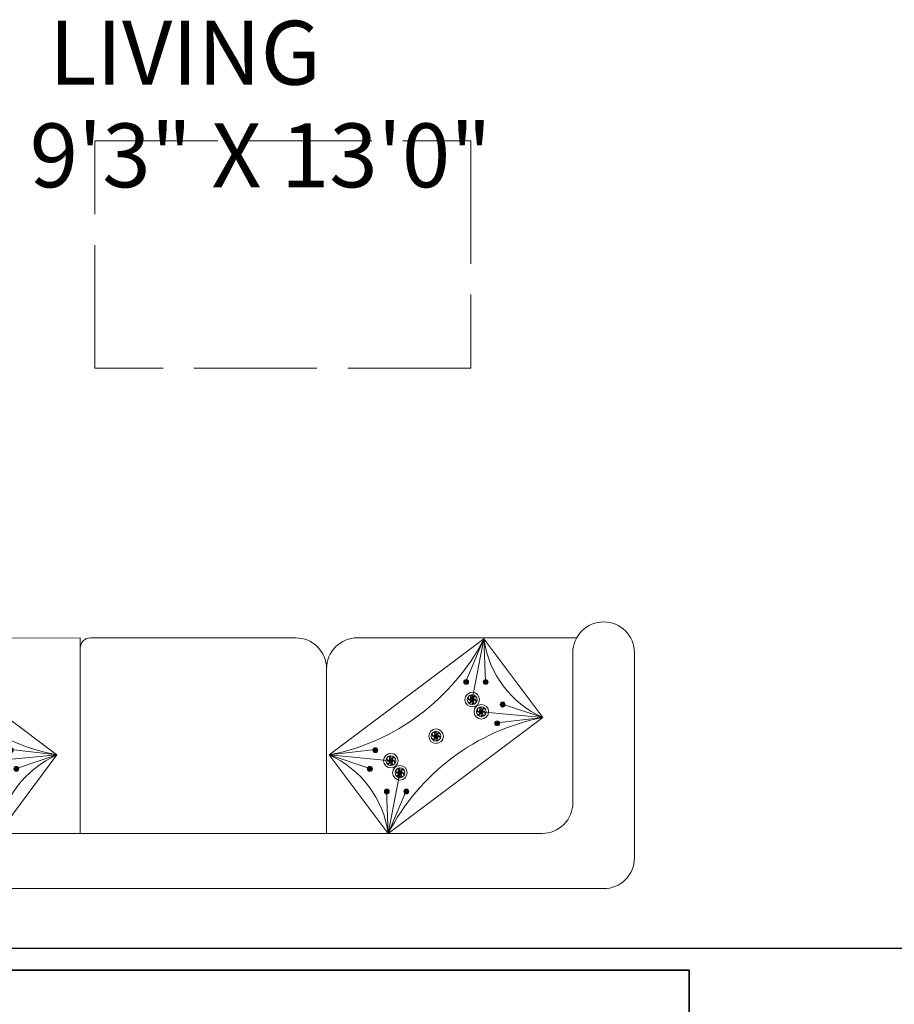
# Model space of a CAD drawing. Units: inches. Extents: x -61 to 1599, y -1316 to 257.
# Tile 194 of 204: x 1147 to 1233, y -173 to -77. Entities that reach past the tile are written whole.
import ezdxf

# ---------------------------------------------------------------- set-up
doc = ezdxf.new("R2010")
doc.units = ezdxf.units.IN
doc.header["$MEASUREMENT"] = 0
doc.linetypes.add('ACAD_ISO02W100', pattern=[15, 12, -3])
for name, color, linetype, lineweight in [('A-ANNO-DIMS', 2, 'Continuous', 18), ('A-AREA-IDEN', 1, 'Continuous', 18), ('A-FURN-LOW', 83, 'ACAD_ISO02W100', 18), ('FURNITURE', 83, 'Continuous', 18), ('WALLS', 4, 'Continuous', 35)]:
    doc.layers.add(name, color=color, linetype=linetype, lineweight=lineweight)
doc.layers.add('FUR', color=83, linetype='Continuous')
doc.styles.get("Standard").update_dxf_attribs({"font": 'arial.ttf'})
doc.dimstyles.get("Standard").update_dxf_attribs({"dimtxt": 0.18, "dimasz": 0.18, "dimexe": 0.18, "dimexo": 0.0625, "dimgap": 0.09, "dimtad": 0, "dimtih": 1, "dimtoh": 1, "dimdec": 0, "dimzin": 0, "dimdsep": 46, "dimlunit": 3, "dimtxsty": 'Standard', "dimcen": 0.09, "dimadec": 0, "dimazin": 0, "dimtfac": 1, "dimtdec": 0, "dimtofl": 0, "dimtmove": 0, "dimatfit": 3, "dimfxl": 1, "dimtolj": 1, "dimtzin": 0, "dimarcsym": 0})

# ---------------------------------------------------------------- blocks, each defined once
blk = doc.blocks.new('*U152')
at = {"layer": 'FUR'}
blk.add_open_spline([(0.005, 0.08), (-0.03, 0.048), (-0.098, -0.015), (0.075, -0.018), (0.024, -0.063), (0.005, -0.08)], degree=3, knots=[0, 0, 0, 0, 0.0954578, 0.1898773, 0.2470677, 0.2470677, 0.2470677, 0.2470677], dxfattribs=at)
blk = doc.blocks.new('*U153')
at = {"layer": 'FUR', "transparency": 16777216}
for p, rotation in [((222.173, -79.977), 60), ((222.178, -80.056), 120), ((222.25, -80.092), 180), ((222.312, -79.968), 300), ((222.317, -80.048), 240)]:
    blk.add_blockref('*U152', p, dxfattribs=dict(at, rotation=rotation))
blk.add_blockref('*U152', (222.24, -79.932), dxfattribs=at)
blk = doc.blocks.new('*U154')
at = {"layer": 'FUR'}
blk.add_open_spline([(0.005, 0.08), (-0.03, 0.048), (-0.098, -0.015), (0.075, -0.018), (0.024, -0.063), (0.005, -0.08)], degree=3, knots=[0, 0, 0, 0, 0.0954578, 0.1898773, 0.2470677, 0.2470677, 0.2470677, 0.2470677], dxfattribs=at)
blk = doc.blocks.new('*U155')
at = {"layer": 'FUR', "transparency": 16777216}
for p, rotation in [((222.173, -79.977), 60), ((222.178, -80.056), 120), ((222.25, -80.092), 180), ((222.312, -79.968), 300), ((222.317, -80.048), 240)]:
    blk.add_blockref('*U154', p, dxfattribs=dict(at, rotation=rotation))
blk.add_blockref('*U154', (222.24, -79.932), dxfattribs=at)
blk = doc.blocks.new('*U148')
at = {"layer": 'FUR'}
blk.add_open_spline([(0.005, 0.08), (-0.03, 0.048), (-0.098, -0.015), (0.075, -0.018), (0.024, -0.063), (0.005, -0.08)], degree=3, knots=[0, 0, 0, 0, 0.0954578, 0.1898773, 0.2470677, 0.2470677, 0.2470677, 0.2470677], dxfattribs=at)
blk = doc.blocks.new('*U149')
at = {"layer": 'FUR', "transparency": 16777216}
for p, rotation in [((222.173, -79.977), 60), ((222.178, -80.056), 120), ((222.25, -80.092), 180), ((222.312, -79.968), 300), ((222.317, -80.048), 240)]:
    blk.add_blockref('*U148', p, dxfattribs=dict(at, rotation=rotation))
blk.add_blockref('*U148', (222.24, -79.932), dxfattribs=at)
blk = doc.blocks.new('*U128')
at = {"layer": 'FUR'}
blk.add_open_spline([(0.015, 0.238), (-0.088, 0.143), (-0.292, -0.045), (0.224, -0.053), (0.072, -0.187), (0.015, -0.238)], degree=3, knots=[0, 0, 0, 0, 0.2846533, 0.5662105, 0.736751, 0.736751, 0.736751, 0.736751], dxfattribs=at)
blk = doc.blocks.new('*U129')
at = {"layer": 'FUR', "transparency": 16777216}
for p, rotation in [((662.517, -238.489), 60), ((662.531, -238.727), 120), ((662.745, -238.833), 180), ((662.929, -238.463), 300), ((662.944, -238.702), 240)]:
    blk.add_blockref('*U128', p, dxfattribs=dict(at, rotation=rotation))
blk.add_blockref('*U128', (662.716, -238.357), dxfattribs=at)
blk = doc.blocks.new('*U150')
at = {"layer": 'FUR'}
blk.add_open_spline([(0.005, 0.08), (-0.03, 0.048), (-0.098, -0.015), (0.075, -0.018), (0.024, -0.063), (0.005, -0.08)], degree=3, knots=[0, 0, 0, 0, 0.0954578, 0.1898773, 0.2470677, 0.2470677, 0.2470677, 0.2470677], dxfattribs=at)
blk = doc.blocks.new('*U151')
at = {"layer": 'FUR', "transparency": 16777216}
for p, rotation in [((222.173, -79.977), 60), ((222.178, -80.056), 120), ((222.25, -80.092), 180), ((222.312, -79.968), 300), ((222.317, -80.048), 240)]:
    blk.add_blockref('*U150', p, dxfattribs=dict(at, rotation=rotation))
blk.add_blockref('*U150', (222.24, -79.932), dxfattribs=at)
blk = doc.blocks.new('*U132')
at = {"layer": 'FUR'}
blk.add_open_spline([(0.015, 0.238), (-0.088, 0.143), (-0.292, -0.045), (0.224, -0.053), (0.072, -0.187), (0.015, -0.238)], degree=3, knots=[0, 0, 0, 0, 0.2846533, 0.5662105, 0.736751, 0.736751, 0.736751, 0.736751], dxfattribs=at)
blk = doc.blocks.new('*U133')
at = {"layer": 'FUR', "transparency": 16777216}
for p, rotation in [((662.517, -238.489), 60), ((662.531, -238.727), 120), ((662.745, -238.833), 180), ((662.929, -238.463), 300), ((662.944, -238.702), 240)]:
    blk.add_blockref('*U132', p, dxfattribs=dict(at, rotation=rotation))
blk.add_blockref('*U132', (662.716, -238.357), dxfattribs=at)
blk = doc.blocks.new('*U124')
at = {"layer": 'FUR'}
blk.add_open_spline([(0.005, 0.08), (-0.03, 0.048), (-0.098, -0.015), (0.075, -0.018), (0.024, -0.063), (0.005, -0.08)], degree=3, knots=[0, 0, 0, 0, 0.0954578, 0.1898773, 0.2470677, 0.2470677, 0.2470677, 0.2470677], dxfattribs=at)
blk = doc.blocks.new('*U125')
at = {"layer": 'FUR', "transparency": 16777216}
for p, rotation in [((222.173, -79.977), 60), ((222.178, -80.056), 120), ((222.25, -80.092), 180), ((222.312, -79.968), 300), ((222.317, -80.048), 240)]:
    blk.add_blockref('*U124', p, dxfattribs=dict(at, rotation=rotation))
blk.add_blockref('*U124', (222.24, -79.932), dxfattribs=at)
blk = doc.blocks.new('*U134')
at = {"layer": 'FUR'}
blk.add_open_spline([(0.015, 0.238), (-0.088, 0.143), (-0.292, -0.045), (0.224, -0.053), (0.072, -0.187), (0.015, -0.238)], degree=3, knots=[0, 0, 0, 0, 0.2846533, 0.5662105, 0.736751, 0.736751, 0.736751, 0.736751], dxfattribs=at)
blk = doc.blocks.new('*U123')
at = {"layer": 'FUR', "transparency": 16777216}
for p, rotation in [((662.517, -238.489), 60), ((662.531, -238.727), 120), ((662.745, -238.833), 180), ((662.929, -238.463), 300), ((662.944, -238.702), 240)]:
    blk.add_blockref('*U134', p, dxfattribs=dict(at, rotation=rotation))
blk.add_blockref('*U134', (662.716, -238.357), dxfattribs=at)
blk = doc.blocks.new('*U130')
at = {"layer": 'FUR'}
blk.add_open_spline([(0.015, 0.238), (-0.088, 0.143), (-0.292, -0.045), (0.224, -0.053), (0.072, -0.187), (0.015, -0.238)], degree=3, knots=[0, 0, 0, 0, 0.2846533, 0.5662105, 0.736751, 0.736751, 0.736751, 0.736751], dxfattribs=at)
blk = doc.blocks.new('*U131')
at = {"layer": 'FUR', "transparency": 16777216}
for p, rotation in [((662.517, -238.489), 60), ((662.531, -238.727), 120), ((662.745, -238.833), 180), ((662.929, -238.463), 300), ((662.944, -238.702), 240)]:
    blk.add_blockref('*U130', p, dxfattribs=dict(at, rotation=rotation))
blk.add_blockref('*U130', (662.716, -238.357), dxfattribs=at)
blk = doc.blocks.new('*U126')
at = {"layer": 'FUR'}
blk.add_open_spline([(0.005, 0.08), (-0.03, 0.048), (-0.098, -0.015), (0.075, -0.018), (0.024, -0.063), (0.005, -0.08)], degree=3, knots=[0, 0, 0, 0, 0.0954578, 0.1898773, 0.2470677, 0.2470677, 0.2470677, 0.2470677], dxfattribs=at)
blk = doc.blocks.new('*U127')
at = {"layer": 'FUR', "transparency": 16777216}
for p, rotation in [((222.173, -79.977), 60), ((222.178, -80.056), 120), ((222.25, -80.092), 180), ((222.312, -79.968), 300), ((222.317, -80.048), 240)]:
    blk.add_blockref('*U126', p, dxfattribs=dict(at, rotation=rotation))
blk.add_blockref('*U126', (222.24, -79.932), dxfattribs=at)
blk = doc.blocks.new('*U146')
at = {"layer": 'FUR'}
blk.add_open_spline([(0.005, 0.08), (-0.03, 0.048), (-0.098, -0.015), (0.075, -0.018), (0.024, -0.063), (0.005, -0.08)], degree=3, knots=[0, 0, 0, 0, 0.0954578, 0.1898773, 0.2470677, 0.2470677, 0.2470677, 0.2470677], dxfattribs=at)
blk = doc.blocks.new('*U147')
at = {"layer": 'FUR', "transparency": 16777216}
for p, rotation in [((222.173, -79.977), 60), ((222.178, -80.056), 120), ((222.25, -80.092), 180), ((222.312, -79.968), 300), ((222.317, -80.048), 240)]:
    blk.add_blockref('*U146', p, dxfattribs=dict(at, rotation=rotation))
blk.add_blockref('*U146', (222.24, -79.932), dxfattribs=at)
blk = doc.blocks.new('*U144')
at = {"layer": 'FUR'}
blk.add_open_spline([(0.005, 0.08), (-0.03, 0.048), (-0.098, -0.015), (0.075, -0.018), (0.024, -0.063), (0.005, -0.08)], degree=3, knots=[0, 0, 0, 0, 0.0954578, 0.1898773, 0.2470677, 0.2470677, 0.2470677, 0.2470677], dxfattribs=at)
blk = doc.blocks.new('*U145')
at = {"layer": 'FUR', "transparency": 16777216}
for p, rotation in [((222.173, -79.977), 60), ((222.178, -80.056), 120), ((222.25, -80.092), 180), ((222.312, -79.968), 300), ((222.317, -80.048), 240)]:
    blk.add_blockref('*U144', p, dxfattribs=dict(at, rotation=rotation))
blk.add_blockref('*U144', (222.24, -79.932), dxfattribs=at)
blk = doc.blocks.new('*U114')
at = {"layer": 'FUR'}
blk.add_open_spline([(0.005, 0.08), (-0.03, 0.048), (-0.098, -0.015), (0.075, -0.018), (0.024, -0.063), (0.005, -0.08)], degree=3, knots=[0, 0, 0, 0, 0.0954578, 0.1898773, 0.2470677, 0.2470677, 0.2470677, 0.2470677], dxfattribs=at)
blk = doc.blocks.new('*U115')
at = {"layer": 'FUR', "transparency": 16777216}
for p, rotation in [((222.173, -79.977), 60), ((222.178, -80.056), 120), ((222.25, -80.092), 180), ((222.312, -79.968), 300), ((222.317, -80.048), 240)]:
    blk.add_blockref('*U114', p, dxfattribs=dict(at, rotation=rotation))
blk.add_blockref('*U114', (222.24, -79.932), dxfattribs=at)
blk = doc.blocks.new('*U116')
at = {"layer": 'FUR'}
blk.add_open_spline([(0.005, 0.08), (-0.03, 0.048), (-0.098, -0.015), (0.075, -0.018), (0.024, -0.063), (0.005, -0.08)], degree=3, knots=[0, 0, 0, 0, 0.0954578, 0.1898773, 0.2470677, 0.2470677, 0.2470677, 0.2470677], dxfattribs=at)
blk = doc.blocks.new('*U117')
at = {"layer": 'FUR', "transparency": 16777216}
for p, rotation in [((222.173, -79.977), 60), ((222.178, -80.056), 120), ((222.25, -80.092), 180), ((222.312, -79.968), 300), ((222.317, -80.048), 240)]:
    blk.add_blockref('*U116', p, dxfattribs=dict(at, rotation=rotation))
blk.add_blockref('*U116', (222.24, -79.932), dxfattribs=at)
blk = doc.blocks.new('*U112')
at = {"layer": 'FUR'}
blk.add_open_spline([(0.005, 0.08), (-0.03, 0.048), (-0.098, -0.015), (0.075, -0.018), (0.024, -0.063), (0.005, -0.08)], degree=3, knots=[0, 0, 0, 0, 0.0954578, 0.1898773, 0.2470677, 0.2470677, 0.2470677, 0.2470677], dxfattribs=at)
blk = doc.blocks.new('*U113')
at = {"layer": 'FUR', "transparency": 16777216}
for p, rotation in [((222.173, -79.977), 60), ((222.178, -80.056), 120), ((222.25, -80.092), 180), ((222.312, -79.968), 300), ((222.317, -80.048), 240)]:
    blk.add_blockref('*U112', p, dxfattribs=dict(at, rotation=rotation))
blk.add_blockref('*U112', (222.24, -79.932), dxfattribs=at)
blk = doc.blocks.new('*U142')
at = {"layer": 'FUR'}
blk.add_open_spline([(0.015, 0.238), (-0.088, 0.143), (-0.292, -0.045), (0.224, -0.053), (0.072, -0.187), (0.015, -0.238)], degree=3, knots=[0, 0, 0, 0, 0.2846533, 0.5662105, 0.736751, 0.736751, 0.736751, 0.736751], dxfattribs=at)
blk = doc.blocks.new('*U143')
at = {"layer": 'FUR', "transparency": 16777216}
for p, rotation in [((662.517, -238.489), 60), ((662.531, -238.727), 120), ((662.745, -238.833), 180), ((662.929, -238.463), 300), ((662.944, -238.702), 240)]:
    blk.add_blockref('*U142', p, dxfattribs=dict(at, rotation=rotation))
blk.add_blockref('*U142', (662.716, -238.357), dxfattribs=at)
blk = doc.blocks.new('*U158')
at = {"layer": 'FUR'}
blk.add_open_spline([(0.015, 0.238), (-0.088, 0.143), (-0.292, -0.045), (0.224, -0.053), (0.072, -0.187), (0.015, -0.238)], degree=3, knots=[0, 0, 0, 0, 0.2846533, 0.5662105, 0.736751, 0.736751, 0.736751, 0.736751], dxfattribs=at)
blk = doc.blocks.new('*U109')
at = {"layer": 'FUR', "transparency": 16777216}
for p, rotation in [((662.517, -238.489), 60), ((662.531, -238.727), 120), ((662.745, -238.833), 180), ((662.929, -238.463), 300), ((662.944, -238.702), 240)]:
    blk.add_blockref('*U158', p, dxfattribs=dict(at, rotation=rotation))
blk.add_blockref('*U158', (662.716, -238.357), dxfattribs=at)
blk = doc.blocks.new('*U110')
at = {"layer": 'FUR'}
blk.add_open_spline([(0.005, 0.08), (-0.03, 0.048), (-0.098, -0.015), (0.075, -0.018), (0.024, -0.063), (0.005, -0.08)], degree=3, knots=[0, 0, 0, 0, 0.0954578, 0.1898773, 0.2470677, 0.2470677, 0.2470677, 0.2470677], dxfattribs=at)
blk = doc.blocks.new('*U111')
at = {"layer": 'FUR', "transparency": 16777216}
for p, rotation in [((222.173, -79.977), 60), ((222.178, -80.056), 120), ((222.25, -80.092), 180), ((222.312, -79.968), 300), ((222.317, -80.048), 240)]:
    blk.add_blockref('*U110', p, dxfattribs=dict(at, rotation=rotation))
blk.add_blockref('*U110', (222.24, -79.932), dxfattribs=at)
blk = doc.blocks.new('*U156')
at = {"layer": 'FUR'}
blk.add_open_spline([(0.015, 0.238), (-0.088, 0.143), (-0.292, -0.045), (0.224, -0.053), (0.072, -0.187), (0.015, -0.238)], degree=3, knots=[0, 0, 0, 0, 0.2846533, 0.5662105, 0.736751, 0.736751, 0.736751, 0.736751], dxfattribs=at)
blk = doc.blocks.new('*U157')
at = {"layer": 'FUR', "transparency": 16777216}
for p, rotation in [((662.517, -238.489), 60), ((662.531, -238.727), 120), ((662.745, -238.833), 180), ((662.929, -238.463), 300), ((662.944, -238.702), 240)]:
    blk.add_blockref('*U156', p, dxfattribs=dict(at, rotation=rotation))
blk.add_blockref('*U156', (662.716, -238.357), dxfattribs=at)
blk = doc.blocks.new('*U120')
at = {"layer": 'FUR'}
blk.add_open_spline([(0.005, 0.08), (-0.03, 0.048), (-0.098, -0.015), (0.075, -0.018), (0.024, -0.063), (0.005, -0.08)], degree=3, knots=[0, 0, 0, 0, 0.0954578, 0.1898773, 0.2470677, 0.2470677, 0.2470677, 0.2470677], dxfattribs=at)
blk = doc.blocks.new('*U121')
at = {"layer": 'FUR', "transparency": 16777216}
for p, rotation in [((222.173, -79.977), 60), ((222.178, -80.056), 120), ((222.25, -80.092), 180), ((222.312, -79.968), 300), ((222.317, -80.048), 240)]:
    blk.add_blockref('*U120', p, dxfattribs=dict(at, rotation=rotation))
blk.add_blockref('*U120', (222.24, -79.932), dxfattribs=at)
blk = doc.blocks.new('*U140')
at = {"layer": 'FUR'}
blk.add_open_spline([(0.015, 0.238), (-0.088, 0.143), (-0.292, -0.045), (0.224, -0.053), (0.072, -0.187), (0.015, -0.238)], degree=3, knots=[0, 0, 0, 0, 0.2846533, 0.5662105, 0.736751, 0.736751, 0.736751, 0.736751], dxfattribs=at)
blk = doc.blocks.new('*U141')
at = {"layer": 'FUR', "transparency": 16777216}
for p, rotation in [((662.517, -238.489), 60), ((662.531, -238.727), 120), ((662.745, -238.833), 180), ((662.929, -238.463), 300), ((662.944, -238.702), 240)]:
    blk.add_blockref('*U140', p, dxfattribs=dict(at, rotation=rotation))
blk.add_blockref('*U140', (662.716, -238.357), dxfattribs=at)
blk = doc.blocks.new('*U135')
at = {"layer": 'FUR'}
blk.add_open_spline([(0.015, 0.238), (-0.088, 0.143), (-0.292, -0.045), (0.224, -0.053), (0.072, -0.187), (0.015, -0.238)], degree=3, knots=[0, 0, 0, 0, 0.2846533, 0.5662105, 0.736751, 0.736751, 0.736751, 0.736751], dxfattribs=at)
blk = doc.blocks.new('*U136')
at = {"layer": 'FUR', "transparency": 16777216}
for p, rotation in [((662.517, -238.489), 60), ((662.531, -238.727), 120), ((662.745, -238.833), 180), ((662.929, -238.463), 300), ((662.944, -238.702), 240)]:
    blk.add_blockref('*U135', p, dxfattribs=dict(at, rotation=rotation))
blk.add_blockref('*U135', (662.716, -238.357), dxfattribs=at)
blk = doc.blocks.new('*U118')
at = {"layer": 'FUR'}
blk.add_open_spline([(0.005, 0.08), (-0.03, 0.048), (-0.098, -0.015), (0.075, -0.018), (0.024, -0.063), (0.005, -0.08)], degree=3, knots=[0, 0, 0, 0, 0.0954578, 0.1898773, 0.2470677, 0.2470677, 0.2470677, 0.2470677], dxfattribs=at)
blk = doc.blocks.new('*U119')
at = {"layer": 'FUR', "transparency": 16777216}
for p, rotation in [((222.173, -79.977), 60), ((222.178, -80.056), 120), ((222.25, -80.092), 180), ((222.312, -79.968), 300), ((222.317, -80.048), 240)]:
    blk.add_blockref('*U118', p, dxfattribs=dict(at, rotation=rotation))
blk.add_blockref('*U118', (222.24, -79.932), dxfattribs=at)
blk = doc.blocks.new('*U138')
at = {"layer": 'FUR'}
blk.add_open_spline([(0.005, 0.08), (-0.03, 0.048), (-0.098, -0.015), (0.075, -0.018), (0.024, -0.063), (0.005, -0.08)], degree=3, knots=[0, 0, 0, 0, 0.0954578, 0.1898773, 0.2470677, 0.2470677, 0.2470677, 0.2470677], dxfattribs=at)
blk = doc.blocks.new('*U139')
at = {"layer": 'FUR', "transparency": 16777216}
for p, rotation in [((222.173, -79.977), 60), ((222.178, -80.056), 120), ((222.25, -80.092), 180), ((222.312, -79.968), 300), ((222.317, -80.048), 240)]:
    blk.add_blockref('*U138', p, dxfattribs=dict(at, rotation=rotation))
blk.add_blockref('*U138', (222.24, -79.932), dxfattribs=at)
blk = doc.blocks.new('*U122')
at = {"layer": 'FUR'}
blk.add_open_spline([(0.005, 0.08), (-0.03, 0.048), (-0.098, -0.015), (0.075, -0.018), (0.024, -0.063), (0.005, -0.08)], degree=3, knots=[0, 0, 0, 0, 0.0954578, 0.1898773, 0.2470677, 0.2470677, 0.2470677, 0.2470677], dxfattribs=at)
blk = doc.blocks.new('*U137')
at = {"layer": 'FUR', "transparency": 16777216}
for p, rotation in [((222.173, -79.977), 60), ((222.178, -80.056), 120), ((222.25, -80.092), 180), ((222.312, -79.968), 300), ((222.317, -80.048), 240)]:
    blk.add_blockref('*U122', p, dxfattribs=dict(at, rotation=rotation))
blk.add_blockref('*U122', (222.24, -79.932), dxfattribs=at)
blk = doc.blocks.new('SOFA-THREE-SEAT')
for p, q in [((30, 24.442), (6.996, 24.38)), ((12.664, 24.333), (12.509, 20.192)), ((12.664, 24.333), (13.805, 18.423)), ((12.664, 24.333), (14.414, 20.192)), ((30, 23.442), (29.997, 24.442)), ((51, 24.442), (31, 24.442)), ((78.369, 24.442), (57, 24.442)), ((69.336, 24.333), (67.586, 20.192)), ((69.336, 24.333), (68.194, 18.423)), ((69.336, 24.333), (69.49, 20.192)), ((6, 23), (5.999, 23.377)), ((30, 23.442), (30, 5.382)), ((54, 21.442), (54, 5.382)), ((54, 21.442), (54, 21.442)), ((12.49, 20.139), (12.49, 20.299)), ((14.394, 20.139), (14.394, 20.299)), ((67.605, 20.139), (67.605, 20.299)), ((69.509, 20.139), (69.509, 20.299)), ((12.49, 20.139), (12.49, 19.979)), ((14.394, 20.139), (14.394, 19.979)), ((67.605, 20.139), (67.605, 19.979)), ((69.509, 20.139), (69.509, 19.979)), ((13.805, 18.423), (13.805, 18.899)), ((13.805, 18.423), (13.805, 17.946)), ((68.194, 18.423), (68.194, 18.899)), ((68.194, 18.423), (68.194, 17.946)), ((6.926, 16.687), (10.859, 17.993)), ((10.84, 17.94), (10.84, 18.1)), ((10.84, 17.94), (10.84, 17.78)), ((69.079, 17.243), (69.079, 17.719)), ((75.074, 16.687), (71.14, 17.993)), ((71.159, 17.94), (71.159, 18.1)), ((71.159, 17.94), (71.159, 17.78)), ((6.926, 16.687), (12.92, 17.243)), ((6.926, 16.687), (11.391, 16.164)), ((75.074, 16.687), (69.079, 17.243)), ((69.079, 17.243), (69.079, 16.766)), ((75.074, 16.687), (70.608, 16.164)), ((11.372, 16.112), (11.372, 16.272)), ((11.372, 16.112), (11.372, 15.952)), ((70.627, 16.112), (70.627, 16.272)), ((70.627, 16.112), (70.627, 15.952)), ((17.327, 14.857), (17.327, 15.334)), ((17.327, 14.857), (17.327, 14.381)), ((64.672, 14.857), (64.672, 15.334)), ((64.672, 14.857), (64.672, 14.381)), ((23.243, 13.498), (23.243, 13.658)), ((23.243, 13.498), (23.243, 13.338)), ((27.729, 13.028), (23.263, 13.551)), ((54.271, 13.028), (58.736, 13.551)), ((58.756, 13.498), (58.756, 13.658)), ((58.756, 13.498), (58.756, 13.338)), ((27.729, 13.028), (21.735, 12.472)), ((21.735, 12.472), (21.735, 12.949)), ((27.729, 13.028), (23.795, 11.722)), ((54.271, 13.028), (60.265, 12.472)), ((54.271, 13.028), (58.204, 11.722)), ((60.265, 12.472), (60.265, 12.949)), ((20.849, 11.292), (20.849, 11.769)), ((21.735, 12.472), (21.735, 11.996)), ((23.776, 11.67), (23.776, 11.83)), ((23.776, 11.67), (23.776, 11.51)), ((58.224, 11.67), (58.224, 11.83)), ((58.224, 11.67), (58.224, 11.51)), ((60.265, 12.472), (60.265, 11.996)), ((61.15, 11.292), (61.15, 11.769)), ((21.991, 5.382), (20.849, 11.292)), ((20.849, 11.292), (20.849, 10.816)), ((60.009, 5.382), (61.15, 11.292)), ((61.15, 11.292), (61.15, 10.816)), ((20.221, 9.471), (20.221, 9.631)), ((22.125, 9.471), (22.125, 9.631)), ((59.874, 9.471), (59.874, 9.631)), ((61.778, 9.471), (61.778, 9.631)), ((20.221, 9.471), (20.221, 9.311)), ((21.991, 5.382), (20.241, 9.523)), ((21.991, 5.382), (22.145, 9.523)), ((22.125, 9.471), (22.125, 9.311)), ((60.009, 5.382), (59.854, 9.523)), ((59.874, 9.471), (59.874, 9.311)), ((60.009, 5.382), (61.759, 9.523)), ((61.778, 9.471), (61.778, 9.311))]:
    blk.add_line(p, q)
blk.add_lwpolyline([(78, 8.382), (78, 23, -0.414214), (81, 26), (81, 26, -0.414214), (84, 23), (84, 3, -0.414214), (81, 0), (3, 0, -0.414214), (0, 3), (0, 23, -0.414214), (3, 26), (3, 26, -0.414214), (6, 23), (6, 8.382, 0.414214), (9, 5.382), (75, 5.382, 0.414214)], format="xyb", close=True)
for points in [[(27.729, 13.028), (12.664, 24.333), (6.926, 16.687), (21.991, 5.382)], [(54.271, 13.028), (69.336, 24.333), (75.074, 16.687), (60.009, 5.382)]]:
    blk.add_lwpolyline(points, close=True)
for centre, radius in [((12.49, 20.139), 0.238), ((12.49, 20.139), 0.16), ((14.394, 20.139), 0.238), ((14.394, 20.139), 0.16), ((67.605, 20.139), 0.238), ((67.605, 20.139), 0.16), ((69.509, 20.139), 0.238), ((69.509, 20.139), 0.16), ((13.805, 18.423), 0.71), ((13.805, 18.423), 0.476), ((68.194, 18.423), 0.71), ((68.194, 18.423), 0.476), ((10.84, 17.94), 0.238), ((10.84, 17.94), 0.16), ((69.079, 17.243), 0.71), ((69.079, 17.243), 0.476), ((71.159, 17.94), 0.238), ((71.159, 17.94), 0.16), ((11.372, 16.112), 0.238), ((70.627, 16.112), 0.238), ((11.372, 16.112), 0.16), ((17.327, 14.857), 0.71), ((64.672, 14.857), 0.71), ((70.627, 16.112), 0.16), ((17.327, 14.857), 0.476), ((64.672, 14.857), 0.476), ((23.243, 13.498), 0.238), ((23.243, 13.498), 0.16), ((58.756, 13.498), 0.238), ((58.756, 13.498), 0.16), ((21.735, 12.472), 0.71), ((21.735, 12.472), 0.476), ((60.265, 12.472), 0.71), ((60.265, 12.472), 0.476), ((20.849, 11.292), 0.71), ((20.849, 11.292), 0.476), ((23.776, 11.67), 0.238), ((23.776, 11.67), 0.16), ((58.224, 11.67), 0.238), ((58.224, 11.67), 0.16), ((61.15, 11.292), 0.71), ((61.15, 11.292), 0.476), ((20.221, 9.471), 0.238), ((20.221, 9.471), 0.16), ((22.125, 9.471), 0.238), ((22.125, 9.471), 0.16), ((59.874, 9.471), 0.238), ((59.874, 9.471), 0.16), ((61.778, 9.471), 0.238), ((61.778, 9.471), 0.16)]:
    blk.add_circle(centre, radius)
for centre, radius, start, end in [((6.999, 23.38), 1, 90.15417, 180.15417), ((2.937, 25.656), 9.816, 293.97422, 352.25297), ((31.951, 34.345), 21.731, 207.43163, 258.79556), ((31, 23.442), 1, 89.99998, 179.99998), ((51, 21.442), 3, 359.99998, 89.99998), ((57, 21.442), 3, 90, 180.00002), ((50.048, 34.345), 21.731, 281.20444, 332.56837), ((79.062, 25.656), 9.816, 187.74703, 246.02578), ((2.703, -4.63), 21.731, 27.43163, 78.79556), ((79.296, -4.63), 21.731, 101.20444, 152.56837), ((31.717, 4.059), 9.816, 113.97422, 172.25297), ((50.282, 4.059), 9.816, 7.74703, 66.02578)]:
    blk.add_arc(centre, radius, start, end)
at = {"xscale": -1, "rotation": 180}
for name, p in [('*U149', (-209.755, -59.873)), ('*U151', (-207.851, -59.873)), ('*U129', (-648.925, -220.172)), ('*U153', (-211.405, -62.072)), ('*U155', (-210.873, -63.9)), ('*U133', (-645.403, -223.738)), ('*U147', (-199.001, -66.514)), ('*U131', (-640.996, -226.123)), ('*U123', (-641.881, -227.303)), ('*U145', (-198.469, -68.342)), ('*U125', (-202.024, -70.541)), ('*U127', (-200.12, -70.541))]:
    blk.add_blockref(name, p, dxfattribs=at)
at = {"rotation": 180}
for name, p in [('*U121', (289.85, -59.873)), ('*U119', (291.754, -59.873)), ('*U141', (730.924, -220.172)), ('*U136', (731.81, -221.352)), ('*U137', (293.404, -62.072)), ('*U139', (292.872, -63.9)), ('*U157', (727.402, -223.738)), ('*U117', (281.001, -66.514)), ('*U143', (722.995, -226.123)), ('*U115', (280.469, -68.342)), ('*U109', (723.88, -227.303)), ('*U113', (282.119, -70.541)), ('*U111', (284.023, -70.541))]:
    blk.add_blockref(name, p, dxfattribs=at)
blk = doc.blocks.new('*D698')
at = {"layer": 'A-ANNO-DIMS', "color": 0, "lineweight": -2, "transparency": 16777216}
for p, q in [((644.765, -167.169), (1598.483, -167.169)), ((1598.303, -167.349), (1598.303, -363.987)), ((1598.303, -560.989), (1598.303, -364.351)), ((644.765, -561.169), (1598.483, -561.169))]:
    blk.add_line(p, q, dxfattribs=at)
at = {"layer": 'A-ANNO-DIMS', "color": 0, "transparency": 16777216}
for points in [[(1598.273, -167.349), (1598.333, -167.349), (1598.303, -167.169)], [(1598.273, -560.989), (1598.333, -560.989), (1598.303, -561.169)]]:
    blk.add_solid(points, dxfattribs=at)
at = {"layer": 'DEFPOINTS', "color": 0, "transparency": 16777216}
for p in [(644.703, -167.169), (1598.303, -167.169), (644.703, -561.169)]:
    blk.add_point(p, dxfattribs=at)
at = {"layer": 'A-ANNO-DIMS', "color": 0, "transparency": 16777216, "insert": (1598.303, -364.169), "char_height": 0.18, "attachment_point": 5}
blk.add_mtext('\\A1;394', dxfattribs=at)

msp = doc.modelspace()

# ---------------------------------------------------------------- linework, layer by layer
at = {"layer": 'A-FURN-LOW'}
msp.add_lwpolyline([(1191.4399, -110.6584), (1154.794, -110.6584), (1154.794, -88.492), (1191.4399, -88.492)], close=True, dxfattribs=at)
at = {"layer": 'WALLS'}
for p in [(1097.7028, -169.3229), (1212.7028, -282.3229)]:
    msp.add_line(p, (1212.7028, -169.3229), dxfattribs=at)

# ---------------------------------------------------------------- block references
at = {"layer": 'FURNITURE'}
msp.add_blockref('SOFA-THREE-SEAT', (1123.375, -161.379), dxfattribs=at)

# ---------------------------------------------------------------- texts
at = {"layer": 'A-AREA-IDEN'}
for s, height, p in [('   LIVING', 6.22364, (1144.6485, -83.0336)), ('  9\'3" X 13\'0"', 6.223643, (1144.6485, -93.0314))]:
    msp.add_text(s, height=height, dxfattribs=at).set_placement(p)

# ---------------------------------------------------------------- dimensions: what is measured, and where the dimension line sits
at = {"layer": 'A-ANNO-DIMS'}
dim = msp.add_linear_dim(base=(1598.3028, -167.169), p1=(644.7028, -561.169), p2=(644.7028, -167.169), angle=90, dimstyle='Standard', override={"dimdec": 0, "dimlfac": 1, "dimrnd": 0, "dimzin": 0, "dimdsep": 46, "dimlunit": 2}, dxfattribs=at)
dim.commit()
dim.dimension.update_dxf_attribs({"geometry": '*D698', "text_midpoint": (1598.3028, -364.169)})

doc.saveas('drawing.dxf')
